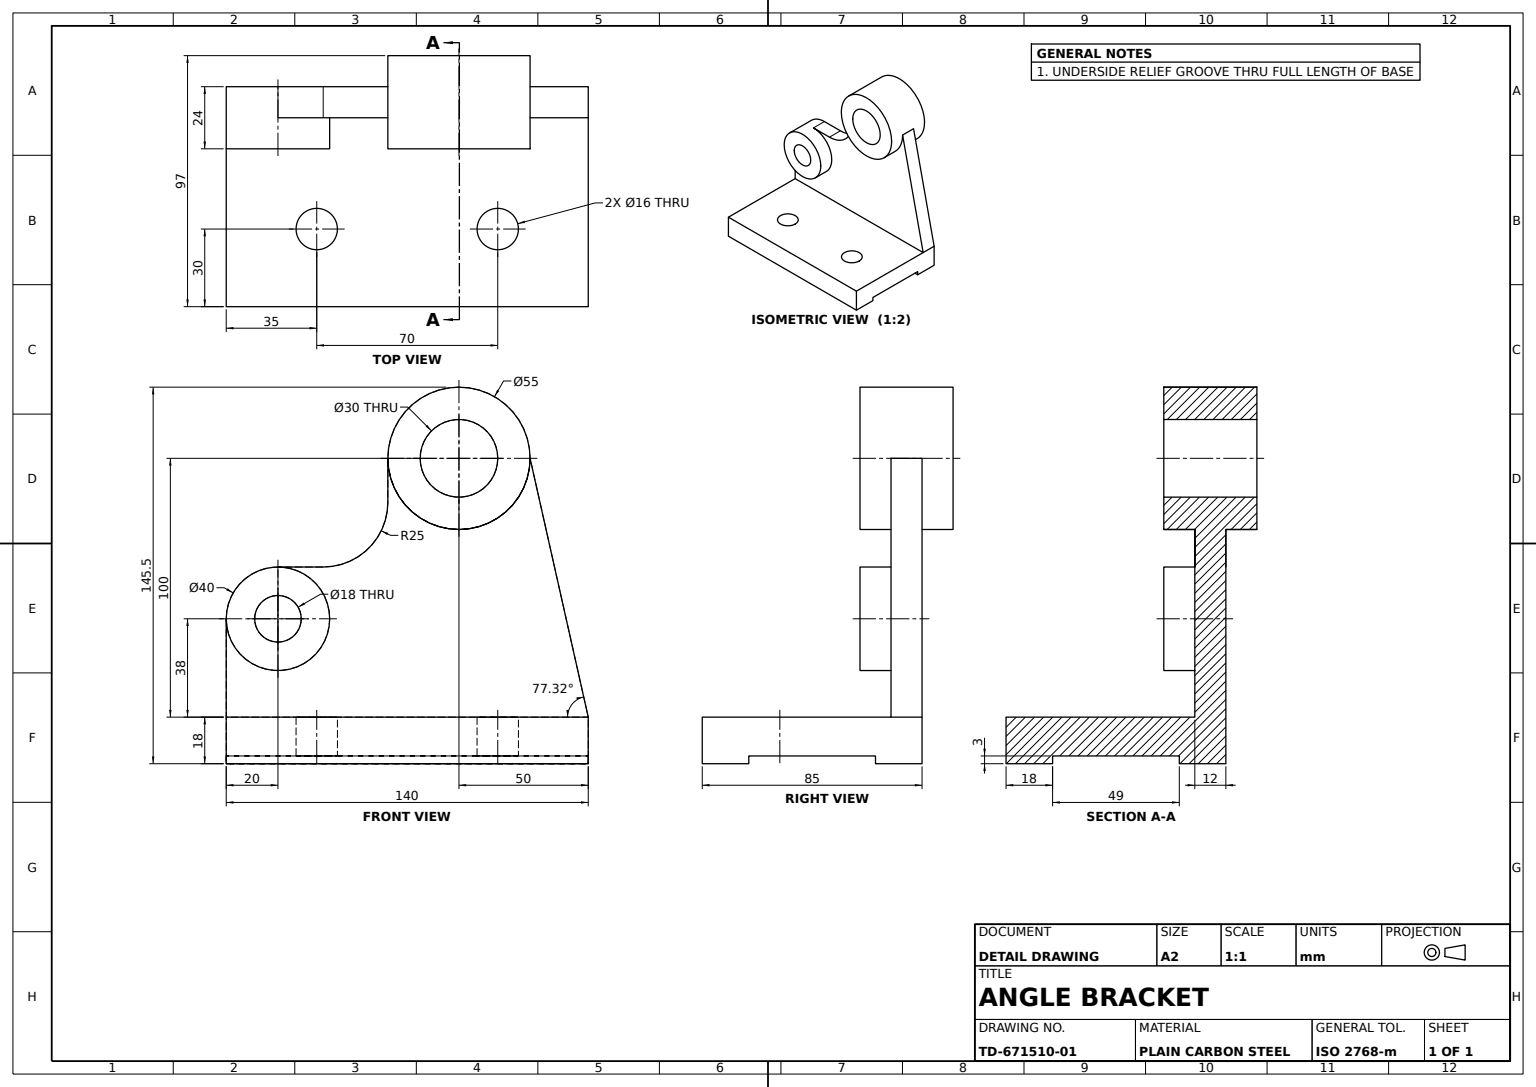
SolidWorks part; units mm, degrees
material "Plain Carbon Steel"
ref_plane "Front Plane" through (0, 0, 0) normal (0, 0, 1) x (1, 0, 0)
ref_plane "Top Plane" through (0, 0, 0) normal (0, 1, 0) x (1, 0, 0)
ref_plane "Right Plane" through (0, 0, 0) normal (1, 0, 0) x (0, 0, -1)
sketch "Base Plate Sketch" plane through (0, 0, 0) normal (0, 1, 0) x (1, 0, 0)
  line L1 (-42.5, 70) -> (42.5, 70)
  line L2 (-42.5, 70) -> (-42.5, -70)
  line L3 (-42.5, -70) -> (42.5, -70)
  line L4 (42.5, 70) -> (42.5, -70)
  line L5 (-42.5, 70) -> (42.5, -70) construction
  line L6 (-42.5, -70) -> (42.5, 70) construction
  point P0 (0, 0)
  dimension "D1" = 140
  dimension "D2" = 85
extrude "Base Plate 140x85x18" add sketch "Base Plate Sketch" along normal blind 18
sketch "Underside Relief Groove Sketch" plane through (0, 0, 70) normal (0, 0, 1) x (1, 0, 0)
  line L0 (42.5, 18) -> (42.5, 0) construction
  line L1 (-42.5, 0) -> (42.5, 0) construction
  line L2 (-24.5, 0) -> (-24.5, 3)
  line L3 (-24.5, 3) -> (24.5, 3)
  line L5 (24.5, 0) -> (24.5, 3)
  line L6 (-24.5, 0) -> (24.5, 0)
  dimension "D1" = 3
  dimension "D2" = 49
  dimension "D3" = 18
extrude "Underside Relief Groove" cut sketch "Underside Relief Groove Sketch" against normal blind 150
sketch "Angled Support Web Sketch" plane through (-42.5, 0, 0) normal (-1, 0, 0) x (0, 0, 1)
  line L0 (70, 18) -> (-70, 18) construction
  line L1 (70, 18) -> (70, 0) construction
  line L2 (-70, 18) -> (-70, 0) construction
  line L3 (70, 18) -> (-70, 18)
  line L4 (-70, 18) -> (-47.5, 118)
  line L5 (70, 18) -> (70, 56)
  line L6 (50, 76) -> (32.5, 76)
  line L7 (7.5, 118) -> (7.5, 101)
  circle A0 centre (50, 56) radius 9
  circle A1 centre (50, 56) radius 20
  circle A2 centre (-20, 118) radius 15
  circle A3 centre (-20, 118) radius 27.5
  arc A4 (32.5, 76) -> (7.5, 101) centre (32.5, 101) cw
  line M6 (70, 18) -> (-70, 18)
  dimension "D1" = 18
  dimension "D2" = 40
  dimension "D5" = 30
  dimension "D6" = 55
  dimension "D9" = 25
  dimension "D3" = 38
  dimension "D4" = 20
  dimension "D7" = 100
  dimension "D8" = 50
extrude "Angled Support Web" add sketch "Angled Support Web Sketch" against normal blind 12 contours L6 A4 L7 A3 L4 L5 A1 M6 | A1 A0 | A3 A2
sketch "Upper Boss Sketch" plane through (-30.5, 0, 0) normal (1, 0, 0) x (0, 0, -1)
  circle A0 centre (-50, 56) radius 9
  circle A1 centre (-50, 56) radius 20
  dimension "D1" = 40
  dimension "D2" = 18
extrude "Upper Boss Ø40" add sketch "Upper Boss Sketch" along normal blind 12
sketch "Lower Boss Sketch A" plane through (-42.5, 0, 0) normal (-1, 0, 0) x (0, 0, 1)
  circle A0 centre (-20, 118) radius 15
  circle A1 centre (-20, 118) radius 27.5
  dimension "D1" = 30
  dimension "D2" = 55
extrude "Lower Boss Ø30 A" add sketch "Lower Boss Sketch A" along normal blind 12
sketch "Lower Boss Sketch B" plane through (-30.5, 0, 0) normal (1, 0, 0) x (0, 0, -1)
  circle A0 centre (20, 118) radius 15
  circle A1 centre (20, 118) radius 27.5
  dimension "D1" = 55
  dimension "D2" = 30
extrude "Lower Boss Ø30 B" add sketch "Lower Boss Sketch B" along normal blind 12
sketch "Base Mounting Holes Sketch" plane through (0, 18, 0) normal (0, 1, 0) x (1, 0, 0)
  line L0 (-30.5, -70) -> (42.5, -70) construction
  line L1 (42.5, -70) -> (42.5, 70) construction
  circle A0 centre (12.5, 35) radius 8
  circle A1 centre (12.5, -35) radius 8
  dimension "D1" = 16
  dimension "D2" = 16
  dimension "D3" = 35
  dimension "D4" = 30
  dimension "D5" = 30
  dimension "D6" = 70
extrude "Base Mounting Holes 2xØ16" cut sketch "Base Mounting Holes Sketch" against normal blind 20
